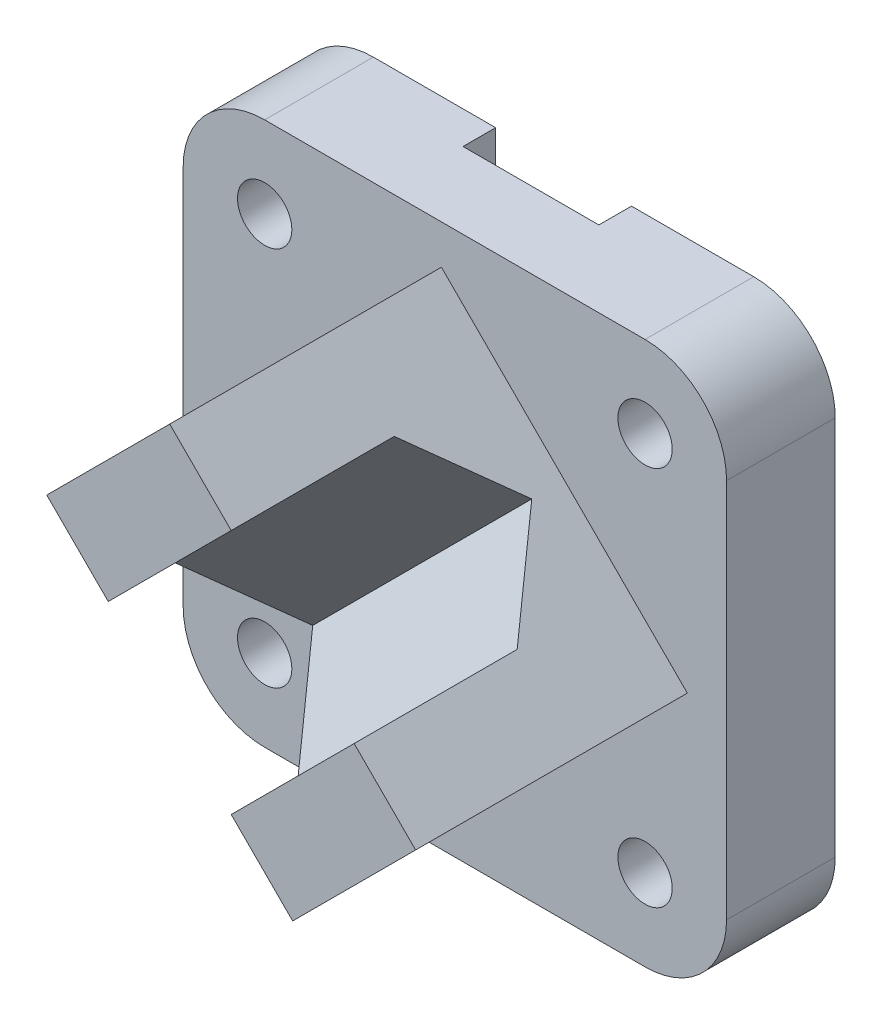
ISO-10303-21;
HEADER;
FILE_DESCRIPTION(('STEP AP214'),'2;1');
FILE_NAME('part.step','',(''),(''),'','','');
FILE_SCHEMA(('AUTOMOTIVE_DESIGN { 1 0 10303 214 1 1 1 1 }'));
ENDSEC;
DATA;
#1=APPLICATION_CONTEXT('core data for automotive mechanical design processes');
#2=APPLICATION_PROTOCOL_DEFINITION('international standard','automotive_design',2000,#1);
#3=PRODUCT_CONTEXT('',#1,'mechanical');
#4=PRODUCT('Part','Part','',(#3));
#5=PRODUCT_RELATED_PRODUCT_CATEGORY('part','',(#4));
#6=PRODUCT_DEFINITION_FORMATION('','',#4);
#7=PRODUCT_DEFINITION_CONTEXT('part definition',#1,'design');
#8=PRODUCT_DEFINITION('design','',#6,#7);
#9=PRODUCT_DEFINITION_SHAPE('','',#8);
#10=(LENGTH_UNIT() NAMED_UNIT(*) SI_UNIT(.MILLI.,.METRE.));
#11=(NAMED_UNIT(*) PLANE_ANGLE_UNIT() SI_UNIT($,.RADIAN.));
#12=(NAMED_UNIT(*) SI_UNIT($,.STERADIAN.) SOLID_ANGLE_UNIT());
#13=UNCERTAINTY_MEASURE_WITH_UNIT(LENGTH_MEASURE(1.E-05),#10,'distance_accuracy_value','');
#14=(GEOMETRIC_REPRESENTATION_CONTEXT(3) GLOBAL_UNCERTAINTY_ASSIGNED_CONTEXT((#13)) GLOBAL_UNIT_ASSIGNED_CONTEXT((#10,
#11,#12)) REPRESENTATION_CONTEXT('',''));
#15=CARTESIAN_POINT('',(0.,0.,0.));
#16=DIRECTION('',(0.,0.,1.));
#17=DIRECTION('',(1.,0.,0.));
#18=AXIS2_PLACEMENT_3D('',#15,#16,#17);
#19=CARTESIAN_POINT('',(0.,0.,70.));
#20=DIRECTION('',(0.,0.,1.));
#21=DIRECTION('',(1.,0.,0.));
#22=AXIS2_PLACEMENT_3D('',#19,#20,#21);
#23=PLANE('',#22);
#24=DIRECTION('',(0.707106781186547,-0.707106781186549,0.));
#25=VECTOR('',#24,1.);
#26=CARTESIAN_POINT('',(20.1525432638167,-25.1022907321225,70.));
#27=LINE('',#26,#25);
#28=CARTESIAN_POINT('',(-25.1022907321224,20.1525432638167,70.));
#29=VERTEX_POINT('',#28);
#30=CARTESIAN_POINT('',(-13.7885822331376,8.83883476483191,70.));
#31=VERTEX_POINT('',#30);
#32=EDGE_CURVE('E388',#29,#31,#27,.T.);
#33=ORIENTED_EDGE('',*,*,#32,.T.);
#34=DIRECTION('',(0.707106781186548,0.707106781186546,0.));
#35=VECTOR('',#34,1.);
#36=CARTESIAN_POINT('',(-61.3137084989848,-38.6862915010151,70.));
#37=LINE('',#36,#35);
#38=CARTESIAN_POINT('',(8.8388347648319,31.4662517628014,70.));
#39=VERTEX_POINT('',#38);
#40=EDGE_CURVE('E222',#31,#39,#37,.T.);
#41=ORIENTED_EDGE('',*,*,#40,.T.);
#42=DIRECTION('',(-0.707106781186547,0.707106781186549,0.));
#43=VECTOR('',#42,1.);
#44=CARTESIAN_POINT('',(-2.47487373415277,42.7799602617861,70.));
#45=LINE('',#44,#43);
#46=CARTESIAN_POINT('',(-2.47487373415277,42.7799602617861,70.));
#47=VERTEX_POINT('',#46);
#48=EDGE_CURVE('E247',#39,#47,#45,.T.);
#49=ORIENTED_EDGE('',*,*,#48,.T.);
#50=DIRECTION('',(-0.707106781186551,-0.707106781186544,0.));
#51=VECTOR('',#50,1.);
#52=CARTESIAN_POINT('',(-42.7799602617861,2.47487373415307,70.));
#53=LINE('',#52,#51);
#54=EDGE_CURVE('E253',#47,#29,#53,.T.);
#55=ORIENTED_EDGE('',*,*,#54,.T.);
#56=EDGE_LOOP('',(#33,#41,#49,#55));
#57=FACE_BOUND('',#56,.T.);
#58=ADVANCED_FACE('F41',(#57),#23,.T.);
#59=CARTESIAN_POINT('',(-47.525126265847,52.4748737341531,52.));
#60=DIRECTION('',(0.707106781186546,-0.707106781186549,0.));
#61=DIRECTION('',(0.707106781186549,0.707106781186546,0.));
#62=AXIS2_PLACEMENT_3D('',#59,#60,#61);
#63=CYLINDRICAL_SURFACE('',#62,8.);
#64=CARTESIAN_POINT('',(-8.83883476483178,13.7885822331377,52.));
#65=DIRECTION('',(-0.707106781186546,0.707106781186548,0.));
#66=DIRECTION('',(-0.707106781186549,-0.707106781186546,0.));
#67=AXIS2_PLACEMENT_3D('',#64,#65,#66);
#68=CIRCLE('',#67,8.);
#69=CARTESIAN_POINT('',(-14.4956890143242,8.13172798364537,52.));
#70=VERTEX_POINT('',#69);
#71=EDGE_CURVE('E234',#70,#70,#68,.F.);
#72=ORIENTED_EDGE('',*,*,#71,.T.);
#73=EDGE_LOOP('',(#72));
#74=FACE_BOUND('',#73,.T.);
#75=CARTESIAN_POINT('',(-20.1525432638165,25.1022907321225,52.));
#76=DIRECTION('',(0.707106781186544,-0.707106781186551,0.));
#77=DIRECTION('',(0.707106781186551,0.707106781186544,0.));
#78=AXIS2_PLACEMENT_3D('',#75,#76,#77);
#79=CIRCLE('',#78,8.);
#80=CARTESIAN_POINT('',(-14.4956890143241,30.7591449816149,52.));
#81=VERTEX_POINT('',#80);
#82=EDGE_CURVE('E239',#81,#81,#79,.T.);
#83=ORIENTED_EDGE('',*,*,#82,.F.);
#84=EDGE_LOOP('',(#83));
#85=FACE_BOUND('',#84,.T.);
#86=ADVANCED_FACE('F447',(#74,#85),#63,.F.);
#87=CARTESIAN_POINT('',(-2.47487373415287,-2.47487373415287,70.));
#88=DIRECTION('',(-0.500000000000001,-0.5,0.707106781186546));
#89=DIRECTION('',(-0.707106781186547,0.707106781186549,0.));
#90=AXIS2_PLACEMENT_3D('',#87,#88,#89);
#91=PLANE('',#90);
#92=DIRECTION('',(-0.5,-0.499999999999999,-0.707106781186549));
#93=VECTOR('',#92,1.);
#94=CARTESIAN_POINT('',(-13.7885822331376,8.83883476483191,70.));
#95=LINE('',#94,#93);
#96=CARTESIAN_POINT('',(-31.4662517628013,-8.83883476483177,44.9999999999999));
#97=VERTEX_POINT('',#96);
#98=EDGE_CURVE('E398',#31,#97,#95,.T.);
#99=ORIENTED_EDGE('',*,*,#98,.F.);
#100=ORIENTED_EDGE('',*,*,#32,.F.);
#101=DIRECTION('',(0.500000000000001,0.499999999999997,0.707106781186549));
#102=VECTOR('',#101,1.);
#103=CARTESIAN_POINT('',(-25.1022907321223,20.1525432638167,70.0000000000001));
#104=LINE('',#103,#102);
#105=CARTESIAN_POINT('',(-42.7799602617861,2.47487373415307,44.9999999999999));
#106=VERTEX_POINT('',#105);
#107=EDGE_CURVE('E397',#106,#29,#104,.T.);
#108=ORIENTED_EDGE('',*,*,#107,.F.);
#109=DIRECTION('',(-0.707106781186547,0.707106781186549,0.));
#110=VECTOR('',#109,1.);
#111=CARTESIAN_POINT('',(-42.7799602617861,2.47487373415308,44.9999999999999));
#112=LINE('',#111,#110);
#113=EDGE_CURVE('E65',#97,#106,#112,.T.);
#114=ORIENTED_EDGE('',*,*,#113,.F.);
#115=EDGE_LOOP('',(#99,#100,#108,#114));
#116=FACE_BOUND('',#115,.T.);
#117=ADVANCED_FACE('F420',(#116),#91,.T.);
#118=CARTESIAN_POINT('',(-35.,-35.,0.));
#119=DIRECTION('',(0.,0.,1.));
#120=DIRECTION('',(1.,0.,0.));
#121=AXIS2_PLACEMENT_3D('',#118,#119,#120);
#122=PLANE('',#121);
#123=CARTESIAN_POINT('',(35.,-35.,0.));
#124=DIRECTION('',(0.,0.,1.));
#125=DIRECTION('',(1.,0.,0.));
#126=AXIS2_PLACEMENT_3D('',#123,#124,#125);
#127=CIRCLE('',#126,5.);
#128=CARTESIAN_POINT('',(40.,-35.,0.));
#129=VERTEX_POINT('',#128);
#130=EDGE_CURVE('E305',#129,#129,#127,.T.);
#131=ORIENTED_EDGE('',*,*,#130,.T.);
#132=EDGE_LOOP('',(#131));
#133=FACE_BOUND('',#132,.T.);
#134=CARTESIAN_POINT('',(35.,35.,0.));
#135=DIRECTION('',(0.,0.,1.));
#136=DIRECTION('',(1.,0.,0.));
#137=AXIS2_PLACEMENT_3D('',#134,#135,#136);
#138=CIRCLE('',#137,5.);
#139=CARTESIAN_POINT('',(40.,35.,0.));
#140=VERTEX_POINT('',#139);
#141=EDGE_CURVE('E306',#140,#140,#138,.T.);
#142=ORIENTED_EDGE('',*,*,#141,.T.);
#143=EDGE_LOOP('',(#142));
#144=FACE_BOUND('',#143,.T.);
#145=DIRECTION('',(1.,0.,0.));
#146=VECTOR('',#145,1.);
#147=CARTESIAN_POINT('',(-34.9999999999999,-50.,0.));
#148=LINE('',#147,#146);
#149=CARTESIAN_POINT('',(12.5,-50.,0.));
#150=VERTEX_POINT('',#149);
#151=CARTESIAN_POINT('',(34.9999999999999,-50.,0.));
#152=VERTEX_POINT('',#151);
#153=EDGE_CURVE('E341',#150,#152,#148,.T.);
#154=ORIENTED_EDGE('',*,*,#153,.F.);
#155=DIRECTION('',(0.,1.,0.));
#156=VECTOR('',#155,1.);
#157=CARTESIAN_POINT('',(12.5,-35.,0.));
#158=LINE('',#157,#156);
#159=CARTESIAN_POINT('',(12.5,50.,0.));
#160=VERTEX_POINT('',#159);
#161=EDGE_CURVE('E293',#150,#160,#158,.T.);
#162=ORIENTED_EDGE('',*,*,#161,.T.);
#163=DIRECTION('',(-1.,0.,0.));
#164=VECTOR('',#163,1.);
#165=CARTESIAN_POINT('',(-34.9999999999999,50.,0.));
#166=LINE('',#165,#164);
#167=CARTESIAN_POINT('',(34.9999999999999,50.,0.));
#168=VERTEX_POINT('',#167);
#169=EDGE_CURVE('E355',#168,#160,#166,.T.);
#170=ORIENTED_EDGE('',*,*,#169,.F.);
#171=CARTESIAN_POINT('',(35.,35.,0.));
#172=DIRECTION('',(0.,0.,1.));
#173=DIRECTION('',(-1.,0.,0.));
#174=AXIS2_PLACEMENT_3D('',#171,#172,#173);
#175=CIRCLE('',#174,15.);
#176=CARTESIAN_POINT('',(50.,34.9999999999999,0.));
#177=VERTEX_POINT('',#176);
#178=EDGE_CURVE('E352',#177,#168,#175,.T.);
#179=ORIENTED_EDGE('',*,*,#178,.F.);
#180=DIRECTION('',(0.,1.,0.));
#181=VECTOR('',#180,1.);
#182=CARTESIAN_POINT('',(50.,34.9999999999999,0.));
#183=LINE('',#182,#181);
#184=CARTESIAN_POINT('',(50.,-34.9999999999999,0.));
#185=VERTEX_POINT('',#184);
#186=EDGE_CURVE('E348',#185,#177,#183,.T.);
#187=ORIENTED_EDGE('',*,*,#186,.F.);
#188=CARTESIAN_POINT('',(35.,-35.,0.));
#189=DIRECTION('',(0.,0.,1.));
#190=DIRECTION('',(1.,0.,0.));
#191=AXIS2_PLACEMENT_3D('',#188,#189,#190);
#192=CIRCLE('',#191,15.);
#193=EDGE_CURVE('E346',#152,#185,#192,.T.);
#194=ORIENTED_EDGE('',*,*,#193,.F.);
#195=EDGE_LOOP('',(#154,#162,#170,#179,#187,#194));
#196=FACE_BOUND('',#195,.T.);
#197=ADVANCED_FACE('F448',(#133,#144,#196),#122,.F.);
#198=CARTESIAN_POINT('',(-34.9999999999999,-50.,20.));
#199=DIRECTION('',(0.,1.,0.));
#200=DIRECTION('',(0.,0.,1.));
#201=AXIS2_PLACEMENT_3D('',#198,#199,#200);
#202=PLANE('',#201);
#203=DIRECTION('',(0.,0.,1.));
#204=VECTOR('',#203,1.);
#205=CARTESIAN_POINT('',(12.5,-50.,-6.));
#206=LINE('',#205,#204);
#207=CARTESIAN_POINT('',(12.5,-50.,6.));
#208=VERTEX_POINT('',#207);
#209=EDGE_CURVE('E273',#150,#208,#206,.T.);
#210=ORIENTED_EDGE('',*,*,#209,.F.);
#211=ORIENTED_EDGE('',*,*,#153,.T.);
#212=DIRECTION('',(0.,0.,-1.));
#213=VECTOR('',#212,1.);
#214=CARTESIAN_POINT('',(34.9999999999999,-50.,20.));
#215=LINE('',#214,#213);
#216=CARTESIAN_POINT('',(34.9999999999999,-50.,20.));
#217=VERTEX_POINT('',#216);
#218=EDGE_CURVE('E378',#217,#152,#215,.T.);
#219=ORIENTED_EDGE('',*,*,#218,.F.);
#220=DIRECTION('',(1.,0.,0.));
#221=VECTOR('',#220,1.);
#222=CARTESIAN_POINT('',(-34.9999999999999,-50.,20.));
#223=LINE('',#222,#221);
#224=CARTESIAN_POINT('',(-34.9999999999999,-50.,20.));
#225=VERTEX_POINT('',#224);
#226=EDGE_CURVE('E326',#225,#217,#223,.T.);
#227=ORIENTED_EDGE('',*,*,#226,.F.);
#228=DIRECTION('',(0.,0.,-1.));
#229=VECTOR('',#228,1.);
#230=CARTESIAN_POINT('',(-34.9999999999999,-50.,20.));
#231=LINE('',#230,#229);
#232=CARTESIAN_POINT('',(-34.9999999999999,-50.,0.));
#233=VERTEX_POINT('',#232);
#234=EDGE_CURVE('E276',#225,#233,#231,.T.);
#235=ORIENTED_EDGE('',*,*,#234,.T.);
#236=CARTESIAN_POINT('',(-12.5,-50.,0.));
#237=VERTEX_POINT('',#236);
#238=EDGE_CURVE('E343',#233,#237,#148,.T.);
#239=ORIENTED_EDGE('',*,*,#238,.T.);
#240=DIRECTION('',(0.,0.,-1.));
#241=VECTOR('',#240,1.);
#242=CARTESIAN_POINT('',(-12.5,-50.,-6.));
#243=LINE('',#242,#241);
#244=CARTESIAN_POINT('',(-12.5,-50.,6.));
#245=VERTEX_POINT('',#244);
#246=EDGE_CURVE('E283',#245,#237,#243,.T.);
#247=ORIENTED_EDGE('',*,*,#246,.F.);
#248=DIRECTION('',(-1.,0.,0.));
#249=VECTOR('',#248,1.);
#250=CARTESIAN_POINT('',(-12.5,-50.,6.));
#251=LINE('',#250,#249);
#252=EDGE_CURVE('E383',#208,#245,#251,.T.);
#253=ORIENTED_EDGE('',*,*,#252,.F.);
#254=EDGE_LOOP('',(#210,#211,#219,#227,#235,#239,#247,#253));
#255=FACE_BOUND('',#254,.T.);
#256=ADVANCED_FACE('F503',(#255),#202,.F.);
#257=CARTESIAN_POINT('',(-35.,-35.,20.));
#258=DIRECTION('',(0.,0.,1.));
#259=DIRECTION('',(1.,0.,0.));
#260=AXIS2_PLACEMENT_3D('',#257,#258,#259);
#261=PLANE('',#260);
#262=DIRECTION('',(0.707106781186547,-0.707106781186549,0.));
#263=VECTOR('',#262,1.);
#264=CARTESIAN_POINT('',(-42.7799602617861,2.47487373415307,20.));
#265=LINE('',#264,#263);
#266=CARTESIAN_POINT('',(-42.7799602617861,2.47487373415307,20.));
#267=VERTEX_POINT('',#266);
#268=CARTESIAN_POINT('',(2.47487373415295,-42.7799602617862,20.));
#269=VERTEX_POINT('',#268);
#270=EDGE_CURVE('E244',#267,#269,#265,.T.);
#271=ORIENTED_EDGE('',*,*,#270,.F.);
#272=DIRECTION('',(-0.707106781186551,-0.707106781186544,0.));
#273=VECTOR('',#272,1.);
#274=CARTESIAN_POINT('',(-42.7799602617861,2.47487373415307,20.));
#275=LINE('',#274,#273);
#276=CARTESIAN_POINT('',(-2.47487373415277,42.7799602617861,20.));
#277=VERTEX_POINT('',#276);
#278=EDGE_CURVE('E250',#277,#267,#275,.T.);
#279=ORIENTED_EDGE('',*,*,#278,.F.);
#280=DIRECTION('',(-0.707106781186547,0.707106781186549,0.));
#281=VECTOR('',#280,1.);
#282=CARTESIAN_POINT('',(-2.47487373415277,42.7799602617861,20.));
#283=LINE('',#282,#281);
#284=CARTESIAN_POINT('',(42.7799602617862,-2.47487373415302,20.));
#285=VERTEX_POINT('',#284);
#286=EDGE_CURVE('E257',#285,#277,#283,.T.);
#287=ORIENTED_EDGE('',*,*,#286,.F.);
#288=DIRECTION('',(0.707106781186549,0.707106781186546,0.));
#289=VECTOR('',#288,1.);
#290=CARTESIAN_POINT('',(2.47487373415295,-42.7799602617862,20.));
#291=LINE('',#290,#289);
#292=EDGE_CURVE('E260',#269,#285,#291,.T.);
#293=ORIENTED_EDGE('',*,*,#292,.F.);
#294=EDGE_LOOP('',(#271,#279,#287,#293));
#295=FACE_BOUND('',#294,.T.);
#296=CARTESIAN_POINT('',(35.,-35.,20.));
#297=DIRECTION('',(0.,0.,1.));
#298=DIRECTION('',(1.,0.,0.));
#299=AXIS2_PLACEMENT_3D('',#296,#297,#298);
#300=CIRCLE('',#299,5.);
#301=CARTESIAN_POINT('',(40.,-35.,20.));
#302=VERTEX_POINT('',#301);
#303=EDGE_CURVE('E303',#302,#302,#300,.T.);
#304=ORIENTED_EDGE('',*,*,#303,.F.);
#305=EDGE_LOOP('',(#304));
#306=FACE_BOUND('',#305,.T.);
#307=CARTESIAN_POINT('',(-35.,35.,20.));
#308=DIRECTION('',(0.,0.,1.));
#309=DIRECTION('',(1.,0.,0.));
#310=AXIS2_PLACEMENT_3D('',#307,#308,#309);
#311=CIRCLE('',#310,5.);
#312=CARTESIAN_POINT('',(-30.,35.,20.));
#313=VERTEX_POINT('',#312);
#314=EDGE_CURVE('E320',#313,#313,#311,.T.);
#315=ORIENTED_EDGE('',*,*,#314,.F.);
#316=EDGE_LOOP('',(#315));
#317=FACE_BOUND('',#316,.T.);
#318=CARTESIAN_POINT('',(-35.,-35.,20.));
#319=DIRECTION('',(0.,0.,1.));
#320=DIRECTION('',(1.,0.,0.));
#321=AXIS2_PLACEMENT_3D('',#318,#319,#320);
#322=CIRCLE('',#321,15.);
#323=CARTESIAN_POINT('',(-50.,-34.9999999999999,20.));
#324=VERTEX_POINT('',#323);
#325=EDGE_CURVE('E323',#324,#225,#322,.T.);
#326=ORIENTED_EDGE('',*,*,#325,.T.);
#327=ORIENTED_EDGE('',*,*,#226,.T.);
#328=CARTESIAN_POINT('',(35.,-35.,20.));
#329=DIRECTION('',(0.,0.,1.));
#330=DIRECTION('',(1.,0.,0.));
#331=AXIS2_PLACEMENT_3D('',#328,#329,#330);
#332=CIRCLE('',#331,15.);
#333=CARTESIAN_POINT('',(50.,-34.9999999999999,20.));
#334=VERTEX_POINT('',#333);
#335=EDGE_CURVE('E328',#217,#334,#332,.T.);
#336=ORIENTED_EDGE('',*,*,#335,.T.);
#337=DIRECTION('',(0.,1.,0.));
#338=VECTOR('',#337,1.);
#339=CARTESIAN_POINT('',(50.,34.9999999999999,20.));
#340=LINE('',#339,#338);
#341=CARTESIAN_POINT('',(50.,34.9999999999999,20.));
#342=VERTEX_POINT('',#341);
#343=EDGE_CURVE('E332',#334,#342,#340,.T.);
#344=ORIENTED_EDGE('',*,*,#343,.T.);
#345=CARTESIAN_POINT('',(35.,35.,20.));
#346=DIRECTION('',(0.,0.,1.));
#347=DIRECTION('',(-1.,0.,0.));
#348=AXIS2_PLACEMENT_3D('',#345,#346,#347);
#349=CIRCLE('',#348,15.);
#350=CARTESIAN_POINT('',(34.9999999999999,50.,20.));
#351=VERTEX_POINT('',#350);
#352=EDGE_CURVE('E334',#342,#351,#349,.T.);
#353=ORIENTED_EDGE('',*,*,#352,.T.);
#354=DIRECTION('',(-1.,0.,0.));
#355=VECTOR('',#354,1.);
#356=CARTESIAN_POINT('',(-34.9999999999999,50.,20.));
#357=LINE('',#356,#355);
#358=CARTESIAN_POINT('',(-34.9999999999999,50.,20.));
#359=VERTEX_POINT('',#358);
#360=EDGE_CURVE('E333',#351,#359,#357,.T.);
#361=ORIENTED_EDGE('',*,*,#360,.T.);
#362=CARTESIAN_POINT('',(-35.,35.,20.));
#363=DIRECTION('',(0.,0.,1.));
#364=DIRECTION('',(1.,0.,0.));
#365=AXIS2_PLACEMENT_3D('',#362,#363,#364);
#366=CIRCLE('',#365,15.);
#367=CARTESIAN_POINT('',(-50.,34.9999999999999,20.));
#368=VERTEX_POINT('',#367);
#369=EDGE_CURVE('E337',#359,#368,#366,.T.);
#370=ORIENTED_EDGE('',*,*,#369,.T.);
#371=DIRECTION('',(0.,-1.,0.));
#372=VECTOR('',#371,1.);
#373=CARTESIAN_POINT('',(-50.,34.9999999999999,20.));
#374=LINE('',#373,#372);
#375=EDGE_CURVE('E338',#368,#324,#374,.T.);
#376=ORIENTED_EDGE('',*,*,#375,.T.);
#377=EDGE_LOOP('',(#326,#327,#336,#344,#353,#361,#370,#376));
#378=FACE_BOUND('',#377,.T.);
#379=CARTESIAN_POINT('',(35.,35.,20.));
#380=DIRECTION('',(0.,0.,1.));
#381=DIRECTION('',(1.,0.,0.));
#382=AXIS2_PLACEMENT_3D('',#379,#380,#381);
#383=CIRCLE('',#382,5.);
#384=CARTESIAN_POINT('',(40.,35.,20.));
#385=VERTEX_POINT('',#384);
#386=EDGE_CURVE('E313',#385,#385,#383,.T.);
#387=ORIENTED_EDGE('',*,*,#386,.F.);
#388=EDGE_LOOP('',(#387));
#389=FACE_BOUND('',#388,.T.);
#390=CARTESIAN_POINT('',(-35.,-35.,20.));
#391=DIRECTION('',(0.,0.,1.));
#392=DIRECTION('',(1.,0.,0.));
#393=AXIS2_PLACEMENT_3D('',#390,#391,#392);
#394=CIRCLE('',#393,5.);
#395=CARTESIAN_POINT('',(-30.,-35.,20.));
#396=VERTEX_POINT('',#395);
#397=EDGE_CURVE('E298',#396,#396,#394,.T.);
#398=ORIENTED_EDGE('',*,*,#397,.F.);
#399=EDGE_LOOP('',(#398));
#400=FACE_BOUND('',#399,.T.);
#401=ADVANCED_FACE('F426',(#295,#306,#317,#378,#389,#400),#261,.T.);
#402=CARTESIAN_POINT('',(-12.5,50.,0.));
#403=VERTEX_POINT('',#402);
#404=CARTESIAN_POINT('',(-34.9999999999999,50.,0.));
#405=VERTEX_POINT('',#404);
#406=EDGE_CURVE('E353',#403,#405,#166,.T.);
#407=ORIENTED_EDGE('',*,*,#406,.F.);
#408=DIRECTION('',(0.,-1.,0.));
#409=VECTOR('',#408,1.);
#410=CARTESIAN_POINT('',(-12.5,-35.,0.));
#411=LINE('',#410,#409);
#412=EDGE_CURVE('E295',#403,#237,#411,.T.);
#413=ORIENTED_EDGE('',*,*,#412,.T.);
#414=ORIENTED_EDGE('',*,*,#238,.F.);
#415=CARTESIAN_POINT('',(-35.,-35.,0.));
#416=DIRECTION('',(0.,0.,1.));
#417=DIRECTION('',(1.,0.,0.));
#418=AXIS2_PLACEMENT_3D('',#415,#416,#417);
#419=CIRCLE('',#418,15.);
#420=CARTESIAN_POINT('',(-50.,-34.9999999999999,0.));
#421=VERTEX_POINT('',#420);
#422=EDGE_CURVE('E319',#421,#233,#419,.T.);
#423=ORIENTED_EDGE('',*,*,#422,.F.);
#424=DIRECTION('',(0.,-1.,0.));
#425=VECTOR('',#424,1.);
#426=CARTESIAN_POINT('',(-50.,34.9999999999999,0.));
#427=LINE('',#426,#425);
#428=CARTESIAN_POINT('',(-50.,34.9999999999999,0.));
#429=VERTEX_POINT('',#428);
#430=EDGE_CURVE('E330',#429,#421,#427,.T.);
#431=ORIENTED_EDGE('',*,*,#430,.F.);
#432=CARTESIAN_POINT('',(-35.,35.,0.));
#433=DIRECTION('',(0.,0.,1.));
#434=DIRECTION('',(1.,0.,0.));
#435=AXIS2_PLACEMENT_3D('',#432,#433,#434);
#436=CIRCLE('',#435,15.);
#437=EDGE_CURVE('E359',#405,#429,#436,.T.);
#438=ORIENTED_EDGE('',*,*,#437,.F.);
#439=EDGE_LOOP('',(#407,#413,#414,#423,#431,#438));
#440=FACE_BOUND('',#439,.T.);
#441=CARTESIAN_POINT('',(-35.,35.,0.));
#442=DIRECTION('',(0.,0.,1.));
#443=DIRECTION('',(1.,0.,0.));
#444=AXIS2_PLACEMENT_3D('',#441,#442,#443);
#445=CIRCLE('',#444,5.);
#446=CARTESIAN_POINT('',(-30.,35.,0.));
#447=VERTEX_POINT('',#446);
#448=EDGE_CURVE('E314',#447,#447,#445,.T.);
#449=ORIENTED_EDGE('',*,*,#448,.T.);
#450=EDGE_LOOP('',(#449));
#451=FACE_BOUND('',#450,.T.);
#452=CARTESIAN_POINT('',(-35.,-35.,0.));
#453=DIRECTION('',(0.,0.,1.));
#454=DIRECTION('',(1.,0.,0.));
#455=AXIS2_PLACEMENT_3D('',#452,#453,#454);
#456=CIRCLE('',#455,5.);
#457=CARTESIAN_POINT('',(-30.,-35.,0.));
#458=VERTEX_POINT('',#457);
#459=EDGE_CURVE('E299',#458,#458,#456,.T.);
#460=ORIENTED_EDGE('',*,*,#459,.T.);
#461=EDGE_LOOP('',(#460));
#462=FACE_BOUND('',#461,.T.);
#463=ADVANCED_FACE('F504',(#440,#451,#462),#122,.F.);
#464=CARTESIAN_POINT('',(-35.,-35.,20.));
#465=DIRECTION('',(0.,0.,-1.));
#466=DIRECTION('',(-1.,0.,0.));
#467=AXIS2_PLACEMENT_3D('',#464,#465,#466);
#468=CYLINDRICAL_SURFACE('',#467,15.);
#469=ORIENTED_EDGE('',*,*,#422,.T.);
#470=ORIENTED_EDGE('',*,*,#234,.F.);
#471=ORIENTED_EDGE('',*,*,#325,.F.);
#472=DIRECTION('',(0.,0.,-1.));
#473=VECTOR('',#472,1.);
#474=CARTESIAN_POINT('',(-50.,-34.9999999999999,20.));
#475=LINE('',#474,#473);
#476=EDGE_CURVE('E342',#324,#421,#475,.T.);
#477=ORIENTED_EDGE('',*,*,#476,.T.);
#478=EDGE_LOOP('',(#469,#470,#471,#477));
#479=FACE_BOUND('',#478,.T.);
#480=ADVANCED_FACE('F510',(#479),#468,.T.);
#481=CARTESIAN_POINT('',(35.,-35.,20.));
#482=DIRECTION('',(0.,0.,-1.));
#483=DIRECTION('',(-1.,0.,0.));
#484=AXIS2_PLACEMENT_3D('',#481,#482,#483);
#485=CYLINDRICAL_SURFACE('',#484,15.);
#486=ORIENTED_EDGE('',*,*,#193,.T.);
#487=DIRECTION('',(0.,0.,-1.));
#488=VECTOR('',#487,1.);
#489=CARTESIAN_POINT('',(50.,-34.9999999999999,20.));
#490=LINE('',#489,#488);
#491=EDGE_CURVE('E374',#334,#185,#490,.T.);
#492=ORIENTED_EDGE('',*,*,#491,.F.);
#493=ORIENTED_EDGE('',*,*,#335,.F.);
#494=ORIENTED_EDGE('',*,*,#218,.T.);
#495=EDGE_LOOP('',(#486,#492,#493,#494));
#496=FACE_BOUND('',#495,.T.);
#497=ADVANCED_FACE('F527',(#496),#485,.T.);
#498=CARTESIAN_POINT('',(50.,34.9999999999999,20.));
#499=DIRECTION('',(-1.,0.,0.));
#500=DIRECTION('',(0.,-1.,0.));
#501=AXIS2_PLACEMENT_3D('',#498,#499,#500);
#502=PLANE('',#501);
#503=ORIENTED_EDGE('',*,*,#186,.T.);
#504=DIRECTION('',(0.,0.,-1.));
#505=VECTOR('',#504,1.);
#506=CARTESIAN_POINT('',(50.,34.9999999999999,20.));
#507=LINE('',#506,#505);
#508=EDGE_CURVE('E375',#342,#177,#507,.T.);
#509=ORIENTED_EDGE('',*,*,#508,.F.);
#510=ORIENTED_EDGE('',*,*,#343,.F.);
#511=ORIENTED_EDGE('',*,*,#491,.T.);
#512=EDGE_LOOP('',(#503,#509,#510,#511));
#513=FACE_BOUND('',#512,.T.);
#514=ADVANCED_FACE('F524',(#513),#502,.F.);
#515=CARTESIAN_POINT('',(35.,35.,20.));
#516=DIRECTION('',(0.,0.,-1.));
#517=DIRECTION('',(-1.,0.,0.));
#518=AXIS2_PLACEMENT_3D('',#515,#516,#517);
#519=CYLINDRICAL_SURFACE('',#518,15.);
#520=ORIENTED_EDGE('',*,*,#178,.T.);
#521=DIRECTION('',(0.,0.,-1.));
#522=VECTOR('',#521,1.);
#523=CARTESIAN_POINT('',(34.9999999999999,50.,20.));
#524=LINE('',#523,#522);
#525=EDGE_CURVE('E369',#351,#168,#524,.T.);
#526=ORIENTED_EDGE('',*,*,#525,.F.);
#527=ORIENTED_EDGE('',*,*,#352,.F.);
#528=ORIENTED_EDGE('',*,*,#508,.T.);
#529=EDGE_LOOP('',(#520,#526,#527,#528));
#530=FACE_BOUND('',#529,.T.);
#531=ADVANCED_FACE('F518',(#530),#519,.T.);
#532=CARTESIAN_POINT('',(-34.9999999999999,50.,20.));
#533=DIRECTION('',(0.,-1.,0.));
#534=DIRECTION('',(0.,0.,-1.));
#535=AXIS2_PLACEMENT_3D('',#532,#533,#534);
#536=PLANE('',#535);
#537=ORIENTED_EDGE('',*,*,#169,.T.);
#538=DIRECTION('',(0.,0.,1.));
#539=VECTOR('',#538,1.);
#540=CARTESIAN_POINT('',(12.5,50.,-6.));
#541=LINE('',#540,#539);
#542=CARTESIAN_POINT('',(12.5,50.,6.));
#543=VERTEX_POINT('',#542);
#544=EDGE_CURVE('E274',#160,#543,#541,.T.);
#545=ORIENTED_EDGE('',*,*,#544,.T.);
#546=DIRECTION('',(-1.,0.,0.));
#547=VECTOR('',#546,1.);
#548=CARTESIAN_POINT('',(-12.5,50.,6.));
#549=LINE('',#548,#547);
#550=CARTESIAN_POINT('',(-12.5,50.,6.));
#551=VERTEX_POINT('',#550);
#552=EDGE_CURVE('E278',#543,#551,#549,.T.);
#553=ORIENTED_EDGE('',*,*,#552,.T.);
#554=DIRECTION('',(0.,0.,-1.));
#555=VECTOR('',#554,1.);
#556=CARTESIAN_POINT('',(-12.5,50.,-6.));
#557=LINE('',#556,#555);
#558=EDGE_CURVE('E284',#551,#403,#557,.T.);
#559=ORIENTED_EDGE('',*,*,#558,.T.);
#560=ORIENTED_EDGE('',*,*,#406,.T.);
#561=DIRECTION('',(0.,0.,-1.));
#562=VECTOR('',#561,1.);
#563=CARTESIAN_POINT('',(-34.9999999999999,50.,20.));
#564=LINE('',#563,#562);
#565=EDGE_CURVE('E368',#359,#405,#564,.T.);
#566=ORIENTED_EDGE('',*,*,#565,.F.);
#567=ORIENTED_EDGE('',*,*,#360,.F.);
#568=ORIENTED_EDGE('',*,*,#525,.T.);
#569=EDGE_LOOP('',(#537,#545,#553,#559,#560,#566,#567,#568));
#570=FACE_BOUND('',#569,.T.);
#571=ADVANCED_FACE('F513',(#570),#536,.F.);
#572=CARTESIAN_POINT('',(-35.,35.,20.));
#573=DIRECTION('',(0.,0.,-1.));
#574=DIRECTION('',(-1.,0.,0.));
#575=AXIS2_PLACEMENT_3D('',#572,#573,#574);
#576=CYLINDRICAL_SURFACE('',#575,15.);
#577=ORIENTED_EDGE('',*,*,#437,.T.);
#578=DIRECTION('',(0.,0.,-1.));
#579=VECTOR('',#578,1.);
#580=CARTESIAN_POINT('',(-50.,34.9999999999999,20.));
#581=LINE('',#580,#579);
#582=EDGE_CURVE('E361',#368,#429,#581,.T.);
#583=ORIENTED_EDGE('',*,*,#582,.F.);
#584=ORIENTED_EDGE('',*,*,#369,.F.);
#585=ORIENTED_EDGE('',*,*,#565,.T.);
#586=EDGE_LOOP('',(#577,#583,#584,#585));
#587=FACE_BOUND('',#586,.T.);
#588=ADVANCED_FACE('F512',(#587),#576,.T.);
#589=CARTESIAN_POINT('',(-50.,34.9999999999999,20.));
#590=DIRECTION('',(1.,0.,0.));
#591=DIRECTION('',(0.,1.,0.));
#592=AXIS2_PLACEMENT_3D('',#589,#590,#591);
#593=PLANE('',#592);
#594=ORIENTED_EDGE('',*,*,#430,.T.);
#595=ORIENTED_EDGE('',*,*,#476,.F.);
#596=ORIENTED_EDGE('',*,*,#375,.F.);
#597=ORIENTED_EDGE('',*,*,#582,.T.);
#598=EDGE_LOOP('',(#594,#595,#596,#597));
#599=FACE_BOUND('',#598,.T.);
#600=ADVANCED_FACE('F496',(#599),#593,.F.);
#601=CARTESIAN_POINT('',(-35.,35.,20.));
#602=DIRECTION('',(0.,0.,-1.));
#603=DIRECTION('',(-1.,0.,0.));
#604=AXIS2_PLACEMENT_3D('',#601,#602,#603);
#605=CYLINDRICAL_SURFACE('',#604,5.);
#606=ORIENTED_EDGE('',*,*,#314,.T.);
#607=EDGE_LOOP('',(#606));
#608=FACE_BOUND('',#607,.T.);
#609=ORIENTED_EDGE('',*,*,#448,.F.);
#610=EDGE_LOOP('',(#609));
#611=FACE_BOUND('',#610,.T.);
#612=ADVANCED_FACE('F494',(#608,#611),#605,.F.);
#613=CARTESIAN_POINT('',(35.,35.,20.));
#614=DIRECTION('',(0.,0.,-1.));
#615=DIRECTION('',(-1.,0.,0.));
#616=AXIS2_PLACEMENT_3D('',#613,#614,#615);
#617=CYLINDRICAL_SURFACE('',#616,5.);
#618=ORIENTED_EDGE('',*,*,#386,.T.);
#619=EDGE_LOOP('',(#618));
#620=FACE_BOUND('',#619,.T.);
#621=ORIENTED_EDGE('',*,*,#141,.F.);
#622=EDGE_LOOP('',(#621));
#623=FACE_BOUND('',#622,.T.);
#624=ADVANCED_FACE('F491',(#620,#623),#617,.F.);
#625=CARTESIAN_POINT('',(35.,-35.,20.));
#626=DIRECTION('',(0.,0.,-1.));
#627=DIRECTION('',(-1.,0.,0.));
#628=AXIS2_PLACEMENT_3D('',#625,#626,#627);
#629=CYLINDRICAL_SURFACE('',#628,5.);
#630=ORIENTED_EDGE('',*,*,#303,.T.);
#631=EDGE_LOOP('',(#630));
#632=FACE_BOUND('',#631,.T.);
#633=ORIENTED_EDGE('',*,*,#130,.F.);
#634=EDGE_LOOP('',(#633));
#635=FACE_BOUND('',#634,.T.);
#636=ADVANCED_FACE('F490',(#632,#635),#629,.F.);
#637=CARTESIAN_POINT('',(-35.,-35.,20.));
#638=DIRECTION('',(0.,0.,-1.));
#639=DIRECTION('',(-1.,0.,0.));
#640=AXIS2_PLACEMENT_3D('',#637,#638,#639);
#641=CYLINDRICAL_SURFACE('',#640,5.);
#642=ORIENTED_EDGE('',*,*,#397,.T.);
#643=EDGE_LOOP('',(#642));
#644=FACE_BOUND('',#643,.T.);
#645=ORIENTED_EDGE('',*,*,#459,.F.);
#646=EDGE_LOOP('',(#645));
#647=FACE_BOUND('',#646,.T.);
#648=ADVANCED_FACE('F483',(#644,#647),#641,.F.);
#649=CARTESIAN_POINT('',(12.5,50.,-6.));
#650=DIRECTION('',(1.,0.,0.));
#651=DIRECTION('',(0.,0.,-1.));
#652=AXIS2_PLACEMENT_3D('',#649,#650,#651);
#653=PLANE('',#652);
#654=ORIENTED_EDGE('',*,*,#209,.T.);
#655=DIRECTION('',(0.,-1.,0.));
#656=VECTOR('',#655,1.);
#657=CARTESIAN_POINT('',(12.5,50.,6.));
#658=LINE('',#657,#656);
#659=EDGE_CURVE('E290',#543,#208,#658,.T.);
#660=ORIENTED_EDGE('',*,*,#659,.F.);
#661=ORIENTED_EDGE('',*,*,#544,.F.);
#662=ORIENTED_EDGE('',*,*,#161,.F.);
#663=EDGE_LOOP('',(#654,#660,#661,#662));
#664=FACE_BOUND('',#663,.T.);
#665=ADVANCED_FACE('F478',(#664),#653,.F.);
#666=CARTESIAN_POINT('',(-12.5,50.,-6.));
#667=DIRECTION('',(-1.,0.,0.));
#668=DIRECTION('',(0.,0.,1.));
#669=AXIS2_PLACEMENT_3D('',#666,#667,#668);
#670=PLANE('',#669);
#671=ORIENTED_EDGE('',*,*,#558,.F.);
#672=DIRECTION('',(0.,-1.,0.));
#673=VECTOR('',#672,1.);
#674=CARTESIAN_POINT('',(-12.5,50.,6.));
#675=LINE('',#674,#673);
#676=EDGE_CURVE('E288',#551,#245,#675,.T.);
#677=ORIENTED_EDGE('',*,*,#676,.T.);
#678=ORIENTED_EDGE('',*,*,#246,.T.);
#679=ORIENTED_EDGE('',*,*,#412,.F.);
#680=EDGE_LOOP('',(#671,#677,#678,#679));
#681=FACE_BOUND('',#680,.T.);
#682=ADVANCED_FACE('F471',(#681),#670,.F.);
#683=CARTESIAN_POINT('',(-12.5,50.,6.));
#684=DIRECTION('',(0.,0.,1.));
#685=DIRECTION('',(1.,0.,0.));
#686=AXIS2_PLACEMENT_3D('',#683,#684,#685);
#687=PLANE('',#686);
#688=ORIENTED_EDGE('',*,*,#676,.F.);
#689=ORIENTED_EDGE('',*,*,#552,.F.);
#690=ORIENTED_EDGE('',*,*,#659,.T.);
#691=ORIENTED_EDGE('',*,*,#252,.T.);
#692=EDGE_LOOP('',(#688,#689,#690,#691));
#693=FACE_BOUND('',#692,.T.);
#694=ADVANCED_FACE('F472',(#693),#687,.F.);
#695=CARTESIAN_POINT('',(-42.7799602617861,2.47487373415307,70.));
#696=DIRECTION('',(0.707106781186549,0.707106781186547,0.));
#697=DIRECTION('',(-0.707106781186547,0.707106781186549,0.));
#698=AXIS2_PLACEMENT_3D('',#695,#696,#697);
#699=PLANE('',#698);
#700=DIRECTION('',(-0.532152084190191,0.532152084190192,0.658504607868518));
#701=VECTOR('',#700,1.);
#702=CARTESIAN_POINT('',(-48.3867538542033,8.08166732657028,60.9380530973452));
#703=LINE('',#702,#701);
#704=CARTESIAN_POINT('',(-20.1525432638166,-20.1525432638165,26.));
#705=VERTEX_POINT('',#704);
#706=CARTESIAN_POINT('',(-31.4662517628013,-8.83883476483176,40.));
#707=VERTEX_POINT('',#706);
#708=EDGE_CURVE('E210',#705,#707,#703,.T.);
#709=ORIENTED_EDGE('',*,*,#708,.T.);
#710=DIRECTION('',(0.,0.,1.));
#711=VECTOR('',#710,1.);
#712=CARTESIAN_POINT('',(-31.4662517628013,-8.83883476483176,70.));
#713=LINE('',#712,#711);
#714=EDGE_CURVE('E232',#707,#97,#713,.T.);
#715=ORIENTED_EDGE('',*,*,#714,.T.);
#716=ORIENTED_EDGE('',*,*,#113,.T.);
#717=DIRECTION('',(0.,0.,-1.));
#718=VECTOR('',#717,1.);
#719=CARTESIAN_POINT('',(-42.7799602617861,2.47487373415307,70.));
#720=LINE('',#719,#718);
#721=EDGE_CURVE('E255',#106,#267,#720,.T.);
#722=ORIENTED_EDGE('',*,*,#721,.T.);
#723=ORIENTED_EDGE('',*,*,#270,.T.);
#724=DIRECTION('',(0.,0.,-1.));
#725=VECTOR('',#724,1.);
#726=CARTESIAN_POINT('',(2.47487373415295,-42.7799602617862,70.));
#727=LINE('',#726,#725);
#728=CARTESIAN_POINT('',(2.47487373415295,-42.7799602617862,44.9999999999999));
#729=VERTEX_POINT('',#728);
#730=EDGE_CURVE('E275',#729,#269,#727,.T.);
#731=ORIENTED_EDGE('',*,*,#730,.F.);
#732=CARTESIAN_POINT('',(-8.83883476483185,-31.4662517628013,44.9999999999999));
#733=VERTEX_POINT('',#732);
#734=EDGE_CURVE('E218',#729,#733,#112,.T.);
#735=ORIENTED_EDGE('',*,*,#734,.T.);
#736=DIRECTION('',(0.,0.,-1.));
#737=VECTOR('',#736,1.);
#738=CARTESIAN_POINT('',(-8.83883476483184,-31.4662517628013,70.));
#739=LINE('',#738,#737);
#740=CARTESIAN_POINT('',(-8.83883476483186,-31.4662517628013,40.));
#741=VERTEX_POINT('',#740);
#742=EDGE_CURVE('E60',#733,#741,#739,.T.);
#743=ORIENTED_EDGE('',*,*,#742,.T.);
#744=DIRECTION('',(-0.532152084190191,0.532152084190192,-0.658504607868518));
#745=VECTOR('',#744,1.);
#746=CARTESIAN_POINT('',(-17.5493890959087,-22.7556974317245,29.221238938053));
#747=LINE('',#746,#745);
#748=EDGE_CURVE('E199',#741,#705,#747,.T.);
#749=ORIENTED_EDGE('',*,*,#748,.T.);
#750=EDGE_LOOP('',(#709,#715,#716,#722,#723,#731,#735,#743,#749));
#751=FACE_BOUND('',#750,.T.);
#752=ADVANCED_FACE('F216',(#751),#699,.F.);
#753=CARTESIAN_POINT('',(2.47487373415295,-42.7799602617862,70.));
#754=DIRECTION('',(-0.707106781186546,0.707106781186549,0.));
#755=DIRECTION('',(-0.707106781186549,-0.707106781186546,0.));
#756=AXIS2_PLACEMENT_3D('',#753,#754,#755);
#757=PLANE('',#756);
#758=CARTESIAN_POINT('',(25.1022907321225,-20.1525432638167,52.));
#759=DIRECTION('',(-0.707106781186546,0.707106781186549,0.));
#760=DIRECTION('',(-0.707106781186549,-0.707106781186546,0.));
#761=AXIS2_PLACEMENT_3D('',#758,#759,#760);
#762=CIRCLE('',#761,8.);
#763=CARTESIAN_POINT('',(19.4454364826301,-25.809397513309,52.));
#764=VERTEX_POINT('',#763);
#765=EDGE_CURVE('E238',#764,#764,#762,.T.);
#766=ORIENTED_EDGE('',*,*,#765,.T.);
#767=EDGE_LOOP('',(#766));
#768=FACE_BOUND('',#767,.T.);
#769=DIRECTION('',(0.707106781186549,0.707106781186546,0.));
#770=VECTOR('',#769,1.);
#771=CARTESIAN_POINT('',(2.47487373415295,-42.7799602617862,70.));
#772=LINE('',#771,#770);
#773=CARTESIAN_POINT('',(20.1525432638167,-25.1022907321225,70.));
#774=VERTEX_POINT('',#773);
#775=CARTESIAN_POINT('',(42.7799602617862,-2.47487373415302,70.));
#776=VERTEX_POINT('',#775);
#777=EDGE_CURVE('E243',#774,#776,#772,.T.);
#778=ORIENTED_EDGE('',*,*,#777,.F.);
#779=DIRECTION('',(-0.5,-0.499999999999998,-0.707106781186549));
#780=VECTOR('',#779,1.);
#781=CARTESIAN_POINT('',(20.1525432638167,-25.1022907321225,70.));
#782=LINE('',#781,#780);
#783=EDGE_CURVE('E394',#774,#729,#782,.T.);
#784=ORIENTED_EDGE('',*,*,#783,.T.);
#785=ORIENTED_EDGE('',*,*,#730,.T.);
#786=ORIENTED_EDGE('',*,*,#292,.T.);
#787=DIRECTION('',(0.,0.,-1.));
#788=VECTOR('',#787,1.);
#789=CARTESIAN_POINT('',(42.7799602617862,-2.47487373415302,70.));
#790=LINE('',#789,#788);
#791=EDGE_CURVE('E267',#776,#285,#790,.T.);
#792=ORIENTED_EDGE('',*,*,#791,.F.);
#793=EDGE_LOOP('',(#778,#784,#785,#786,#792));
#794=FACE_BOUND('',#793,.T.);
#795=ADVANCED_FACE('F431',(#768,#794),#757,.F.);
#796=CARTESIAN_POINT('',(-2.47487373415277,42.7799602617861,70.));
#797=DIRECTION('',(-0.707106781186549,-0.707106781186546,0.));
#798=DIRECTION('',(0.707106781186546,-0.707106781186549,0.));
#799=AXIS2_PLACEMENT_3D('',#796,#797,#798);
#800=PLANE('',#799);
#801=ORIENTED_EDGE('',*,*,#48,.F.);
#802=DIRECTION('',(0.,0.,-1.));
#803=VECTOR('',#802,1.);
#804=CARTESIAN_POINT('',(8.83883476483193,31.4662517628014,70.));
#805=LINE('',#804,#803);
#806=CARTESIAN_POINT('',(8.83883476483192,31.4662517628014,40.));
#807=VERTEX_POINT('',#806);
#808=EDGE_CURVE('E208',#39,#807,#805,.T.);
#809=ORIENTED_EDGE('',*,*,#808,.T.);
#810=DIRECTION('',(0.532152084190191,-0.532152084190192,-0.658504607868518));
#811=VECTOR('',#810,1.);
#812=CARTESIAN_POINT('',(-8.08166732657001,48.3867538542034,60.9380530973451));
#813=LINE('',#812,#811);
#814=CARTESIAN_POINT('',(20.1525432638167,20.1525432638166,26.));
#815=VERTEX_POINT('',#814);
#816=EDGE_CURVE('E11',#807,#815,#813,.T.);
#817=ORIENTED_EDGE('',*,*,#816,.T.);
#818=DIRECTION('',(0.532152084190191,-0.532152084190193,0.658504607868518));
#819=VECTOR('',#818,1.);
#820=CARTESIAN_POINT('',(22.7556974317247,17.5493890959086,29.2212389380531));
#821=LINE('',#820,#819);
#822=CARTESIAN_POINT('',(31.4662517628014,8.8388347648318,40.));
#823=VERTEX_POINT('',#822);
#824=EDGE_CURVE('E49',#815,#823,#821,.T.);
#825=ORIENTED_EDGE('',*,*,#824,.T.);
#826=DIRECTION('',(0.,0.,1.));
#827=VECTOR('',#826,1.);
#828=CARTESIAN_POINT('',(31.4662517628014,8.83883476483182,70.));
#829=LINE('',#828,#827);
#830=CARTESIAN_POINT('',(31.4662517628014,8.83883476483178,70.));
#831=VERTEX_POINT('',#830);
#832=EDGE_CURVE('E215',#823,#831,#829,.T.);
#833=ORIENTED_EDGE('',*,*,#832,.T.);
#834=EDGE_CURVE('E249',#776,#831,#45,.T.);
#835=ORIENTED_EDGE('',*,*,#834,.F.);
#836=ORIENTED_EDGE('',*,*,#791,.T.);
#837=ORIENTED_EDGE('',*,*,#286,.T.);
#838=DIRECTION('',(0.,0.,-1.));
#839=VECTOR('',#838,1.);
#840=CARTESIAN_POINT('',(-2.47487373415277,42.7799602617861,70.));
#841=LINE('',#840,#839);
#842=EDGE_CURVE('E266',#47,#277,#841,.T.);
#843=ORIENTED_EDGE('',*,*,#842,.F.);
#844=EDGE_LOOP('',(#801,#809,#817,#825,#833,#835,#836,#837,#843));
#845=FACE_BOUND('',#844,.T.);
#846=ADVANCED_FACE('F401',(#845),#800,.F.);
#847=CARTESIAN_POINT('',(-42.7799602617861,2.47487373415307,70.));
#848=DIRECTION('',(0.707106781186544,-0.707106781186551,0.));
#849=DIRECTION('',(0.707106781186551,0.707106781186544,0.));
#850=AXIS2_PLACEMENT_3D('',#847,#848,#849);
#851=PLANE('',#850);
#852=ORIENTED_EDGE('',*,*,#82,.T.);
#853=EDGE_LOOP('',(#852));
#854=FACE_BOUND('',#853,.T.);
#855=ORIENTED_EDGE('',*,*,#721,.F.);
#856=ORIENTED_EDGE('',*,*,#107,.T.);
#857=ORIENTED_EDGE('',*,*,#54,.F.);
#858=ORIENTED_EDGE('',*,*,#842,.T.);
#859=ORIENTED_EDGE('',*,*,#278,.T.);
#860=EDGE_LOOP('',(#855,#856,#857,#858,#859));
#861=FACE_BOUND('',#860,.T.);
#862=ADVANCED_FACE('F425',(#854,#861),#851,.F.);
#863=DIRECTION('',(0.707106781186548,0.707106781186546,0.));
#864=VECTOR('',#863,1.);
#865=CARTESIAN_POINT('',(-38.6862915010153,-61.3137084989847,70.));
#866=LINE('',#865,#864);
#867=CARTESIAN_POINT('',(8.83883476483187,-13.7885822331377,70.));
#868=VERTEX_POINT('',#867);
#869=EDGE_CURVE('E213',#868,#831,#866,.T.);
#870=ORIENTED_EDGE('',*,*,#869,.F.);
#871=EDGE_CURVE('E279',#868,#774,#27,.T.);
#872=ORIENTED_EDGE('',*,*,#871,.T.);
#873=ORIENTED_EDGE('',*,*,#777,.T.);
#874=ORIENTED_EDGE('',*,*,#834,.T.);
#875=EDGE_LOOP('',(#870,#872,#873,#874));
#876=FACE_BOUND('',#875,.T.);
#877=ADVANCED_FACE('F432',(#876),#23,.T.);
#878=CARTESIAN_POINT('',(13.7885822331377,-8.83883476483183,52.));
#879=DIRECTION('',(0.707106781186546,-0.707106781186548,0.));
#880=DIRECTION('',(0.707106781186549,0.707106781186546,0.));
#881=AXIS2_PLACEMENT_3D('',#878,#879,#880);
#882=CIRCLE('',#881,8.);
#883=CARTESIAN_POINT('',(19.4454364826301,-3.18198051533946,52.));
#884=VERTEX_POINT('',#883);
#885=EDGE_CURVE('E219',#884,#884,#882,.F.);
#886=ORIENTED_EDGE('',*,*,#885,.T.);
#887=EDGE_LOOP('',(#886));
#888=FACE_BOUND('',#887,.T.);
#889=ORIENTED_EDGE('',*,*,#765,.F.);
#890=EDGE_LOOP('',(#889));
#891=FACE_BOUND('',#890,.T.);
#892=ADVANCED_FACE('F438',(#888,#891),#63,.F.);
#893=DIRECTION('',(0.5,0.499999999999999,0.707106781186549));
#894=VECTOR('',#893,1.);
#895=CARTESIAN_POINT('',(8.83883476483188,-13.7885822331377,70.));
#896=LINE('',#895,#894);
#897=EDGE_CURVE('E399',#733,#868,#896,.T.);
#898=ORIENTED_EDGE('',*,*,#897,.F.);
#899=ORIENTED_EDGE('',*,*,#734,.F.);
#900=ORIENTED_EDGE('',*,*,#783,.F.);
#901=ORIENTED_EDGE('',*,*,#871,.F.);
#902=EDGE_LOOP('',(#898,#899,#900,#901));
#903=FACE_BOUND('',#902,.T.);
#904=ADVANCED_FACE('F42',(#903),#91,.T.);
#905=CARTESIAN_POINT('',(-61.3137084989848,-38.6862915010151,40.));
#906=DIRECTION('',(-0.465633073666417,0.465633073666418,-0.752576694706878));
#907=DIRECTION('',(0.,0.850390405524374,0.526152219601981));
#908=AXIS2_PLACEMENT_3D('',#905,#906,#907);
#909=PLANE('',#908);
#910=DIRECTION('',(0.707106781186548,0.707106781186546,0.));
#911=VECTOR('',#910,1.);
#912=CARTESIAN_POINT('',(-50.0000000000001,-49.9999999999999,26.));
#913=LINE('',#912,#911);
#914=EDGE_CURVE('E202',#705,#815,#913,.T.);
#915=ORIENTED_EDGE('',*,*,#914,.T.);
#916=ORIENTED_EDGE('',*,*,#816,.F.);
#917=DIRECTION('',(0.707106781186548,0.707106781186546,0.));
#918=VECTOR('',#917,1.);
#919=CARTESIAN_POINT('',(-61.3137084989848,-38.6862915010151,40.));
#920=LINE('',#919,#918);
#921=EDGE_CURVE('E226',#707,#807,#920,.T.);
#922=ORIENTED_EDGE('',*,*,#921,.F.);
#923=ORIENTED_EDGE('',*,*,#708,.F.);
#924=EDGE_LOOP('',(#915,#916,#922,#923));
#925=FACE_BOUND('',#924,.T.);
#926=ADVANCED_FACE('F406',(#925),#909,.F.);
#927=CARTESIAN_POINT('',(-38.6862915010153,-61.3137084989847,40.));
#928=DIRECTION('',(0.465633073666416,-0.465633073666418,-0.752576694706878));
#929=DIRECTION('',(0.,0.850390405524374,-0.52615221960198));
#930=AXIS2_PLACEMENT_3D('',#927,#928,#929);
#931=PLANE('',#930);
#932=DIRECTION('',(0.707106781186548,0.707106781186546,0.));
#933=VECTOR('',#932,1.);
#934=CARTESIAN_POINT('',(-38.6862915010153,-61.3137084989847,40.));
#935=LINE('',#934,#933);
#936=EDGE_CURVE('E205',#741,#823,#935,.T.);
#937=ORIENTED_EDGE('',*,*,#936,.T.);
#938=ORIENTED_EDGE('',*,*,#824,.F.);
#939=ORIENTED_EDGE('',*,*,#914,.F.);
#940=ORIENTED_EDGE('',*,*,#748,.F.);
#941=EDGE_LOOP('',(#937,#938,#939,#940));
#942=FACE_BOUND('',#941,.T.);
#943=ADVANCED_FACE('F203',(#942),#931,.F.);
#944=CARTESIAN_POINT('',(-61.3137084989848,-38.6862915010151,70.));
#945=DIRECTION('',(-0.707106781186546,0.707106781186548,0.));
#946=DIRECTION('',(-0.707106781186549,-0.707106781186546,0.));
#947=AXIS2_PLACEMENT_3D('',#944,#945,#946);
#948=PLANE('',#947);
#949=ORIENTED_EDGE('',*,*,#71,.F.);
#950=EDGE_LOOP('',(#949));
#951=FACE_BOUND('',#950,.T.);
#952=ORIENTED_EDGE('',*,*,#40,.F.);
#953=ORIENTED_EDGE('',*,*,#98,.T.);
#954=ORIENTED_EDGE('',*,*,#714,.F.);
#955=ORIENTED_EDGE('',*,*,#921,.T.);
#956=ORIENTED_EDGE('',*,*,#808,.F.);
#957=EDGE_LOOP('',(#952,#953,#954,#955,#956));
#958=FACE_BOUND('',#957,.T.);
#959=ADVANCED_FACE('F415',(#951,#958),#948,.F.);
#960=CARTESIAN_POINT('',(-38.6862915010153,-61.3137084989847,70.));
#961=DIRECTION('',(0.707106781186546,-0.707106781186548,0.));
#962=DIRECTION('',(0.707106781186549,0.707106781186546,0.));
#963=AXIS2_PLACEMENT_3D('',#960,#961,#962);
#964=PLANE('',#963);
#965=ORIENTED_EDGE('',*,*,#885,.F.);
#966=EDGE_LOOP('',(#965));
#967=FACE_BOUND('',#966,.T.);
#968=ORIENTED_EDGE('',*,*,#936,.F.);
#969=ORIENTED_EDGE('',*,*,#742,.F.);
#970=ORIENTED_EDGE('',*,*,#897,.T.);
#971=ORIENTED_EDGE('',*,*,#869,.T.);
#972=ORIENTED_EDGE('',*,*,#832,.F.);
#973=EDGE_LOOP('',(#968,#969,#970,#971,#972));
#974=FACE_BOUND('',#973,.T.);
#975=ADVANCED_FACE('F209',(#967,#974),#964,.F.);
#976=CLOSED_SHELL('',(#58,#86,#117,#197,#256,#401,#463,#480,#497,#514,#531,#571,#588,#600,#612,
#624,#636,#648,#665,#682,#694,#752,#795,#846,#862,#877,#892,#904,#926,#943,#959,#975));
#977=MANIFOLD_SOLID_BREP('B2',#976);
#978=ADVANCED_BREP_SHAPE_REPRESENTATION('',(#18,#977),#14);
#979=SHAPE_DEFINITION_REPRESENTATION(#9,#978);
ENDSEC;
END-ISO-10303-21;
